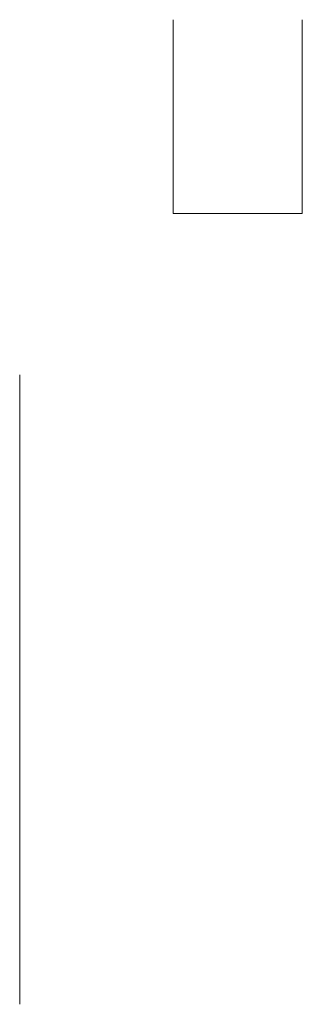
# Model space of a CAD drawing. Units: millimetres. Extents: x 220 to 255, y 700 to 822.
import ezdxf

# ---------------------------------------------------------------- set-up
doc = ezdxf.new("R2010")
doc.units = ezdxf.units.MM
doc.layers.add('M-CONS', color=8, linetype='Continuous', lineweight=13)

msp = doc.modelspace()

# ---------------------------------------------------------------- linework, layer by layer
at = {"layer": 'M-CONS'}
for p, q in [((238.98, 797.79, 34), (238.98, 821.79, 34)), ((254.98, 821.79, 34), (254.98, 797.79, 34)), ((254.98, 797.79, 34), (238.98, 797.79, 34)), ((219.98, 717.79, 22), (219.98, 777.79, 22)), ((219.98, 777.79, 22), (219.98, 777.79, -26)), ((219.98, 739.79, 22), (219.98, 699.79, 22)), ((219.98, 699.79), (219.98, 717.79)), ((219.98, 699.79), (219.98, 717.79)), ((219.98, 717.79), (219.98, 717.79, 22))]:
    msp.add_line(p, q, dxfattribs=at)

doc.saveas('drawing.dxf')
